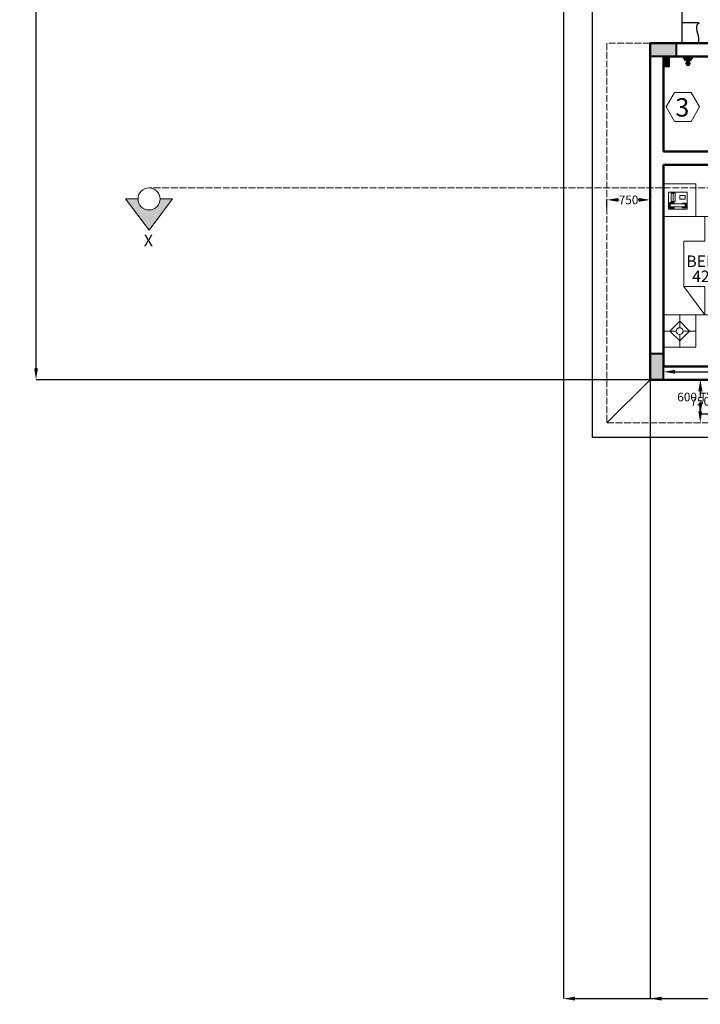
# Model space of a CAD drawing. Units: inches. Extents: x 22626 to 57351, y 2118 to 36234.
# Tile 1 of 10: x 22626 to 34432, y 2118 to 19205. Entities that reach past the tile are written whole.
import ezdxf

# ---------------------------------------------------------------- set-up
doc = ezdxf.new("R2010")
doc.units = ezdxf.units.IN
doc.header["$MEASUREMENT"] = 0
doc.linetypes.add('ACAD_ISO02W100', pattern=[15, 12, -3])
for name, color, linetype, lineweight in [('A-ANNO-DIMS', 130, 'Continuous', 18), ('A-ANNO-SYMB', 130, 'Continuous', 18), ('A-AREA-IDEN', 130, 'Continuous', 18), ('A-COLS', 7, 'Continuous', 40), ('A-FLOR-FIXT', 30, 'Continuous', 18), ('A-ROOF', 80, 'Continuous', 25), ('A-ROOF-OVHD', 80, 'ACAD_ISO02W100', 18), ('A-WALL', 80, 'Continuous', 50), ('FURNITURE', 30, 'Continuous', 18)]:
    doc.layers.add(name, color=color, linetype=linetype, lineweight=lineweight)
doc.layers.add('A-SECT', color=2, linetype='ACAD_ISO02W100', lineweight=18, true_color=0xf1eb1f)
doc.styles.get("Standard").update_dxf_attribs({"font": 'arial.ttf'})
doc.dimstyles.get("Standard").update_dxf_attribs({"dimtxt": 150, "dimasz": 200, "dimexe": 0.18, "dimexo": 0.0625, "dimgap": 0.09, "dimtad": 0, "dimtih": 1, "dimtoh": 1, "dimdec": 0, "dimzin": 0, "dimdsep": 46, "dimtxsty": 'Standard', "dimcen": 0.09, "dimadec": 0, "dimazin": 0, "dimtfac": 1, "dimtdec": 0, "dimtofl": 0, "dimtmove": 0, "dimatfit": 3, "dimfxl": 1, "dimtolj": 1, "dimtzin": 0, "dimarcsym": 0})

# ---------------------------------------------------------------- blocks, each defined once
blk = doc.blocks.new('Phone - Desk')
for p, q in [((-4.5, -5), (-4.5, 5)), ((-4.5, 5), (4.5, 5)), ((-4, 4.5), (-4, 2)), ((-4, 2), (-3.25, 2)), ((-3.75, 4.5), (-3.75, 2.25)), ((-1.25, 4.5), (-3.75, 4.5)), ((-3.75, 2.25), (-3.25, 2.25)), ((-3.25, 4), (-3.25, -4)), ((-3.25, 4), (-1.75, 4)), ((-1.75, -4), (-1.75, 4)), ((-1.75, 2.25), (-1.25, 2.25)), ((-1.75, 2), (-1, 2)), ((-1.25, 2.25), (-1.25, 4.5)), ((-1, 2), (-1, 4.5)), ((4, 3.5), (-0.5, 3.5)), ((-0.5, 3.5), (-0.5, 1.5)), ((-0.5, 2.5), (4, 2.5)), ((-0.5, 1.5), (4, 1.5)), ((4, 1.5), (4, 3.5)), ((4.5, 5), (4.5, -5)), ((4.5, -5), (-4.5, -5)), ((-3.75, -2.25), (-3.25, -2.25)), ((-3.75, -4.5), (-3.75, -2.25)), ((-1.25, -4.5), (-3.75, -4.5)), ((-3.25, -4), (-1.75, -4)), ((-1.75, -2.25), (-1.25, -2.25)), ((-1.25, -2.25), (-1.25, -4.5)), ((2.75, -1), (0.75, -1)), ((0.75, -1), (0.75, -4)), ((0.75, -4), (2.75, -4)), ((2.75, -4), (2.75, -1))]:
    blk.add_line(p, q)
blk = doc.blocks.new('BED')
h = blk.add_hatch()
h.set_pattern_fill('AR-B816', color=256, scale=27, angle=45)
h.paths.add_polyline_path([(36405, 26901), (36405, 25191), (35361, 25191), (35361, 24640), (36931, 24640), (36931, 25191), (36931, 27463), (36405, 27463), (35361, 27463), (35361, 26901)])
for p, q in [((35361, 26901), (35361, 27463)), ((35361, 27463), (36405, 27463)), ((36405, 27463), (36931, 27463)), ((36931, 27463), (36931, 25191)), ((35035, 26901), (35035, 26469)), ((34673, 25686), (34673, 26469)), ((35035, 26469), (34673, 26469)), ((35035, 25686), (34673, 25686)), ((34673, 25686), (35035, 25191)), ((35035, 25191), (35035, 25686)), ((34599, 25191), (34599, 24968)), ((35361, 24640), (35361, 25191)), ((36931, 25191), (36931, 24640)), ((34429, 24909), (34599, 25080)), ((34599, 25080), (34769, 24909)), ((34317, 24909), (34540, 24909)), ((34599, 24739), (34429, 24909)), ((34769, 24909), (34599, 24739)), ((34599, 24850), (34599, 24628)), ((34658, 24909), (34880, 24909)), ((36931, 24640), (35361, 24640))]:
    blk.add_line(p, q)
for points in [[(34317, 26901), (34880, 26901), (34880, 27463), (34317, 27463)], [(34317, 26901), (36405, 26901), (36405, 25191), (34317, 25191)], [(34317, 25191), (34880, 25191), (34880, 24628), (34317, 24628)]]:
    blk.add_lwpolyline(points, close=True)
blk.add_circle((34599, 24909), 59)
at = {"xscale": 32.52267765020765, "yscale": 32.52267765020765, "zscale": 32.52267765020765, "rotation": 90}
blk.add_blockref('Phone - Desk', (34567, 27173), dxfattribs=at)
blk = doc.blocks.new('*D18')
at = {"layer": 'A-ANNO-DIMS', "color": 0, "lineweight": -2, "transparency": 16777216}
for p, q in [((32812, 15954), (32812, 16078)), ((33012, 16078), (33023, 16078)), ((33362, 16078), (33352, 16078)), ((33562, 15954), (33562, 16078))]:
    blk.add_line(p, q, dxfattribs=at)
at = {"layer": 'A-ANNO-DIMS', "color": 0, "transparency": 16777216}
for points in [[(33012, 16111), (33012, 16045), (32812, 16078)], [(33362, 16111), (33362, 16045), (33562, 16078)]]:
    blk.add_solid(points, dxfattribs=at)
at = {"layer": 'Defpoints', "color": 0, "transparency": 16777216}
for p in [(32812, 16078), (32812, 15954), (33562, 15954)]:
    blk.add_point(p, dxfattribs=at)
at = {"layer": 'A-ANNO-DIMS', "color": 0, "transparency": 16777216, "insert": (33187, 16078), "char_height": 150, "attachment_point": 5}
blk.add_mtext('\\A1;750', dxfattribs=at)
blk = doc.blocks.new('*D19')
at = {"layer": 'A-ANNO-DIMS', "color": 0, "lineweight": -2, "transparency": 16777216}
for p, q in [((34431, 12957), (34431, 12957)), ((34431, 12757), (34431, 12659)), ((34431, 12407), (34431, 12505)), ((34431, 12207), (34431, 12207))]:
    blk.add_line(p, q, dxfattribs=at)
at = {"layer": 'A-ANNO-DIMS', "color": 0, "transparency": 16777216}
for points in [[(34398, 12757), (34464, 12757), (34431, 12957)], [(34398, 12407), (34464, 12407), (34431, 12207)]]:
    blk.add_solid(points, dxfattribs=at)
at = {"layer": 'Defpoints', "color": 0, "transparency": 16777216}
for p in [(34431, 12957), (34431, 12207), (34431, 12207)]:
    blk.add_point(p, dxfattribs=at)
at = {"layer": 'A-ANNO-DIMS', "color": 0, "transparency": 16777216, "insert": (34431, 12582), "char_height": 150, "attachment_point": 5}
blk.add_mtext('\\A1;750', dxfattribs=at)
blk = doc.blocks.new('COL-RECTANGULAR')
h = blk.add_hatch(color=256)
h.dxf.hatch_style = 1
h.paths.add_polyline_path([(0, 0), (450, 0), (450, 230), (0, 230)])
blk.add_lwpolyline([(0, 0), (0, 230), (450, 230), (450, 0)], close=True)
blk = doc.blocks.new('SECTION-HEAD')
h = blk.add_hatch(color=256)
h.dxf.hatch_style = 1
h.paths.add_polyline_path([(815, 541), (599, 541, -1), (216, 541), (0, 541), (407, 0)])
for p, q in [((216, 541), (0, 541)), ((0, 541), (407, 0)), ((815, 541), (407, 0)), ((599, 541), (815, 541))]:
    blk.add_line(p, q)
blk.add_circle((407, 541), 191)
blk = doc.blocks.new('CANOPY-EDGE-UNIT')
blk.add_lwpolyline([(0, 355), (300, 355), (300, 0), (0, 0)])
blk.add_open_spline([(0, 0), (4, 58), (10, 128), (45, 238), (49, 340), (0, 355)], degree=3, knots=[0, 0, 0, 0, 169.253843, 206.158158, 361.823024, 361.823024, 361.823024, 361.823024])
blk = doc.blocks.new('BATH-SUPPLY-FITTING')
h = blk.add_hatch(color=256)
h.dxf.hatch_style = 1
h.paths.add_polyline_path([(161, 189), (85, 141), (161, 95)])
h = blk.add_hatch(color=256)
h.dxf.hatch_style = 1
h.paths.add_polyline_path([(161, 95), (58, 125, 1.908564), (58, 64)])
h = blk.add_hatch(color=256)
h.dxf.hatch_style = 1
h.paths.add_polyline_path([(161, 95), (85, 48), (161, 0)])
for p, q in [((161, 189), (85, 141)), ((161, 95), (58, 125)), ((161, 95), (58, 64)), ((85, 141), (161, 95)), ((85, 48), (161, 95)), ((161, 0), (85, 48))]:
    blk.add_line(p, q)
blk.add_arc((37, 95), 37.1, 55.305, 304.695)
blk = doc.blocks.new('BATH-WALL-BOX')
h = blk.add_hatch(color=256)
h.dxf.hatch_style = 1
h.paths.add_polyline_path([(182, 107), (0, 107), (0, 0), (182, 0)])
for p, q in [((0, 0), (0, 107)), ((0, 107), (182, 107)), ((182, 0), (0, 0))]:
    blk.add_line(p, q)
blk = doc.blocks.new('*D61')
at = {"layer": 'A-ANNO-DIMS', "color": 0, "lineweight": -2, "transparency": 16777216}
for p, q in [((33792, 13519), (33792, 13094)), ((36406, 13519), (36406, 13094)), ((33992, 13094), (34616, 13094)), ((36206, 13094), (35582, 13094))]:
    blk.add_line(p, q, dxfattribs=at)
at = {"layer": 'A-ANNO-DIMS', "color": 0, "transparency": 16777216}
for points in [[(33992, 13127), (33992, 13061), (33792, 13094)], [(36206, 13127), (36206, 13061), (36406, 13094)]]:
    blk.add_solid(points, dxfattribs=at)
at = {"layer": 'Defpoints', "color": 0, "transparency": 16777216}
for p in [(33792, 13519), (36406, 13519), (36406, 13094)]:
    blk.add_point(p, dxfattribs=at)
at = {"layer": 'A-ANNO-DIMS', "color": 0, "transparency": 16777216, "insert": (35099, 13094), "char_height": 150, "attachment_point": 5}
blk.add_mtext('\\A1;2613 TYP.', dxfattribs=at)
blk = doc.blocks.new('*D89')
at = {"layer": 'A-ANNO-DIMS', "color": 0, "lineweight": -2, "transparency": 16777216}
for p, q in [((34763, 12957), (34435, 12957)), ((34435, 12757), (34435, 12734)), ((34435, 12557), (34435, 12580)), ((34763, 12357), (34435, 12357))]:
    blk.add_line(p, q, dxfattribs=at)
at = {"layer": 'A-ANNO-DIMS', "color": 0, "transparency": 16777216}
for points in [[(34401, 12757), (34468, 12757), (34435, 12957)], [(34401, 12557), (34468, 12557), (34435, 12357)]]:
    blk.add_solid(points, dxfattribs=at)
at = {"layer": 'Defpoints', "color": 0, "transparency": 16777216}
for p in [(34435, 12957), (34763, 12957), (34763, 12357)]:
    blk.add_point(p, dxfattribs=at)
at = {"layer": 'A-ANNO-DIMS', "color": 0, "transparency": 16777216, "insert": (34435, 12657), "char_height": 150, "attachment_point": 5}
blk.add_mtext('\\A1;600 TYP.', dxfattribs=at)
blk = doc.blocks.new('*D100')
at = {"layer": 'A-ANNO-DIMS', "color": 0, "lineweight": -2, "transparency": 16777216}
for p, q in [((32057, 23297), (32057, 2216)), ((49187, 23297), (49187, 2216)), ((32257, 2216), (40347, 2216)), ((48987, 2216), (40897, 2216))]:
    blk.add_line(p, q, dxfattribs=at)
at = {"layer": 'A-ANNO-DIMS', "color": 0, "transparency": 16777216}
for points in [[(32257, 2250), (32257, 2183), (32057, 2216)], [(48987, 2250), (48987, 2183), (49187, 2216)]]:
    blk.add_solid(points, dxfattribs=at)
at = {"layer": 'Defpoints', "color": 0, "transparency": 16777216}
for p in [(32057, 23297), (49187, 23297), (49187, 2216)]:
    blk.add_point(p, dxfattribs=at)
at = {"layer": 'A-ANNO-DIMS', "color": 0, "transparency": 16777216, "insert": (40622, 2216), "char_height": 150, "attachment_point": 5}
blk.add_mtext('\\A1;17130', dxfattribs=at)
blk = doc.blocks.new('*D101')
at = {"layer": 'A-ANNO-DIMS', "color": 0, "lineweight": -2, "transparency": 16777216}
for p, q in [((31157, 28257), (22910, 28257)), ((22910, 28057), (22910, 20684)), ((22910, 13157), (22910, 20530)), ((33562, 12957), (22910, 12957))]:
    blk.add_line(p, q, dxfattribs=at)
at = {"layer": 'A-ANNO-DIMS', "color": 0, "transparency": 16777216}
for points in [[(22877, 28057), (22943, 28057), (22910, 28257)], [(22877, 13157), (22943, 13157), (22910, 12957)]]:
    blk.add_solid(points, dxfattribs=at)
at = {"layer": 'Defpoints', "color": 0, "transparency": 16777216}
for p in [(31157, 28257), (22910, 12957), (33562, 12957)]:
    blk.add_point(p, dxfattribs=at)
at = {"layer": 'A-ANNO-DIMS', "color": 0, "transparency": 16777216, "insert": (22910, 20607), "char_height": 150, "attachment_point": 5}
blk.add_mtext('\\A1;15300', dxfattribs=at)
blk = doc.blocks.new('*D113')
at = {"layer": 'A-ANNO-DIMS', "color": 0, "lineweight": -2, "transparency": 16777216}
for p, q in [((33562, 12957), (33562, 2216)), ((47682, 12957), (47682, 2216)), ((33762, 2216), (40347, 2216)), ((47482, 2216), (40897, 2216))]:
    blk.add_line(p, q, dxfattribs=at)
at = {"layer": 'A-ANNO-DIMS', "color": 0, "transparency": 16777216}
for points in [[(33762, 2250), (33762, 2183), (33562, 2216)], [(47482, 2250), (47482, 2183), (47682, 2216)]]:
    blk.add_solid(points, dxfattribs=at)
at = {"layer": 'Defpoints', "color": 0, "transparency": 16777216}
for p in [(33562, 12957), (47682, 12957), (47682, 2216)]:
    blk.add_point(p, dxfattribs=at)
at = {"layer": 'A-ANNO-DIMS', "color": 0, "transparency": 16777216, "insert": (40622, 2216), "char_height": 150, "attachment_point": 5}
blk.add_mtext('\\A1;14120', dxfattribs=at)

msp = doc.modelspace()

# ---------------------------------------------------------------- linework, layer by layer
at = {"layer": 'A-AREA-IDEN'}
msp.add_lwpolyline([(34419.43, 17690.31), (34274.22, 17941.81), (33983.81, 17941.81), (33838.61, 17690.31), (33983.81, 17438.81), (34274.22, 17438.81)], close=True, dxfattribs=at)
at = {"layer": 'A-ROOF'}
for p, q in [((34112.43, 23296.86), (34112.43, 18796.86)), ((32812.43, 12206.86), (33562.43, 12956.86))]:
    msp.add_line(p, q, dxfattribs=at)
msp.add_lwpolyline([(43702.43, 11956.86), (43702.43, 7256.86), (37542.43, 7256.86), (37542.43, 11956.86), (32562.43, 11956.86), (32562.43, 22296.86), (30057.43, 22296.86), (30057.43, 24356.86), (30057.43, 30256.86), (39684.53, 30256.86)], dxfattribs=at)
at = {"layer": 'A-ROOF-OVHD', "ltscale": 10}
for p, q in [((33562.43, 18796.86), (32812.43, 18796.86)), ((32812.43, 18796.86), (32812.43, 12206.86)), ((33562.43, 18796.86), (32812.43, 18796.86)), ((32812.43, 18796.86), (32812.43, 12206.86)), ((32812.43, 12206.86), (37992.43, 12206.86)), ((32812.43, 12206.86), (37992.43, 12206.86))]:
    msp.add_line(p, q, dxfattribs=at)
at = {"layer": 'A-SECT', "ltscale": 10}
msp.add_line((55067.61, 16286.11), (24870.06, 16286.11), dxfattribs=at)
at = {"layer": 'A-WALL'}
for p, q in [((36942.43, 18796.86), (33562.43, 18796.86)), ((33562.43, 18796.86), (33562.43, 16916.86)), ((33562.43, 16916.86), (33562.43, 12956.86)), ((36942.43, 16686.86), (33792.43, 16686.86)), ((33792.43, 16686.86), (33792.43, 13186.86)), ((33792.43, 13186.86), (34892.43, 13186.86)), ((33562.43, 12956.86), (38222.43, 12956.86))]:
    msp.add_line(p, q, dxfattribs=at)
for points in [[(36712.43, 16686.86), (36712.43, 18566.86), (33792.43, 18566.86), (33792.43, 16916.86)], [(35817.46, 16916.86), (33792.43, 16916.86)]]:
    msp.add_lwpolyline(points, dxfattribs=at)

# ---------------------------------------------------------------- block references
at = {"layer": 'A-ANNO-SYMB'}
msp.add_blockref('SECTION-HEAD', (24462.57, 15553.84), dxfattribs=at)
at = {"layer": 'A-COLS'}
msp.add_blockref('COL-RECTANGULAR', (33562.43, 18566.86), dxfattribs=at)
at = {"layer": 'A-COLS', "extrusion": (0, 0, -1), "zscale": -1, "rotation": 90}
msp.add_blockref('COL-RECTANGULAR', (-33562.43, 12956.86), dxfattribs=at)
at = {"layer": 'A-FLOR-FIXT', "extrusion": (0, 0, -1), "zscale": -1, "rotation": 90}
for name, p in [('BATH-WALL-BOX', (-33792.43, 18384.84)), ('BATH-SUPPLY-FITTING', (-34123.26, 18405.85))]:
    msp.add_blockref(name, p, dxfattribs=at)
at = {"layer": 'A-ROOF', "extrusion": (0, 0, -1), "zscale": -1}
msp.add_blockref('CANOPY-EDGE-UNIT', (-34412.43, 18796.86), dxfattribs=at)
at = {"layer": 'FURNITURE'}
msp.add_blockref('BED', (-525, -11108.87), dxfattribs=at)

# ---------------------------------------------------------------- texts
at = {"layer": 'A-ANNO-SYMB'}
msp.add_text('X', height=200, dxfattribs=at).set_placement((24781.23, 15273))
at = {"layer": 'A-AREA-IDEN'}
for s, height, p in [('3', 318.67, (33999.46, 17523.63)), ('BED ROOM', 200, (34189.69, 14912.85)), ('4200X3500', 200, (34290.45, 14650.3))]:
    msp.add_text(s, height=height, dxfattribs=at).set_placement(p)

# ---------------------------------------------------------------- dimensions: what is measured, and where the dimension line sits
at = {"layer": 'A-ANNO-DIMS'}
for base, p1, p2, override, picture, middle in [((22910.07, 12956.86), (31157.43, 28256.86), (33562.43, 12956.86), {"dimdec": 0, "dimlfac": 1, "dimrnd": 0, "dimzin": 0, "dimdsep": 46, "dimlunit": 2}, '*D101', (22910.07, 20606.86)), ((34431.02, 12206.86), (34431.02, 12956.86), (34431.02, 12206.86), {"dimclrd": 0, "dimclre": 0, "dimclrt": 0}, '*D19', (34431.02, 12581.86))]:
    dim = msp.add_linear_dim(base=base, p1=p1, p2=p2, angle=90, dimstyle='Standard', override=override, dxfattribs=at)
    dim.commit()
    dim.dimension.update_dxf_attribs({"geometry": picture, "text_midpoint": middle})
for base, p1, p2, override, picture, middle in [((49187.43, 2216.37), (32057.43, 23296.86), (49187.43, 23296.86), {"dimdec": 0, "dimlfac": 1, "dimrnd": 0, "dimzin": 0, "dimdsep": 46, "dimlunit": 2}, '*D100', (40622.43, 2216.37)), ((32812.43, 16078.12), (33562.43, 15953.76), (32812.43, 15953.76), {"dimclrd": 0, "dimclre": 0, "dimclrt": 0}, '*D18', (33187.43, 16078.12)), ((47682.43, 2216.37), (33562.43, 12956.86), (47682.43, 12956.86), {"dimdec": 0, "dimlfac": 1, "dimrnd": 0, "dimzin": 0, "dimdsep": 46, "dimlunit": 2}, '*D113', (40622.43, 2216.37))]:
    dim = msp.add_linear_dim(base=base, p1=p1, p2=p2, dimstyle='Standard', override=override, dxfattribs=at)
    dim.commit()
    dim.dimension.update_dxf_attribs({"geometry": picture, "text_midpoint": middle})
dim = msp.add_linear_dim(base=(36405.75, 13093.9), p1=(33792.43, 13519.2), p2=(36405.75, 13519.2), text='<> TYP.', dimstyle='Standard', override={"dimdec": 0, "dimlfac": 1, "dimrnd": 0, "dimzin": 0, "dimdsep": 46, "dimlunit": 2}, dxfattribs=at)
dim.commit()
dim.dimension.update_dxf_attribs({"geometry": '*D61', "text_midpoint": (35099.09, 13093.9)})
dim = msp.add_linear_dim(base=(34434.79, 12956.86), p1=(34763.36, 12356.86), p2=(34763.36, 12956.86), angle=90, text='<> TYP.', dimstyle='Standard', override={"dimdec": 0, "dimlfac": 1, "dimrnd": 0, "dimzin": 0, "dimdsep": 46, "dimlunit": 2}, dxfattribs=at)
dim.commit()
dim.dimension.update_dxf_attribs({"geometry": '*D89', "text_midpoint": (34434.79, 12656.86)})

doc.saveas('drawing.dxf')
